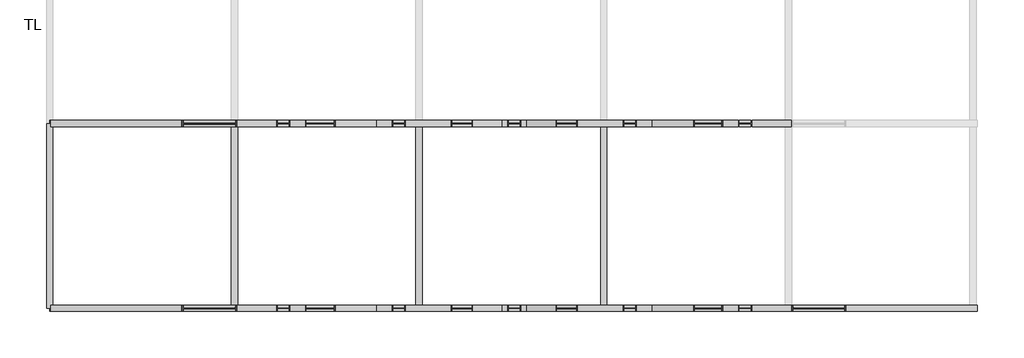
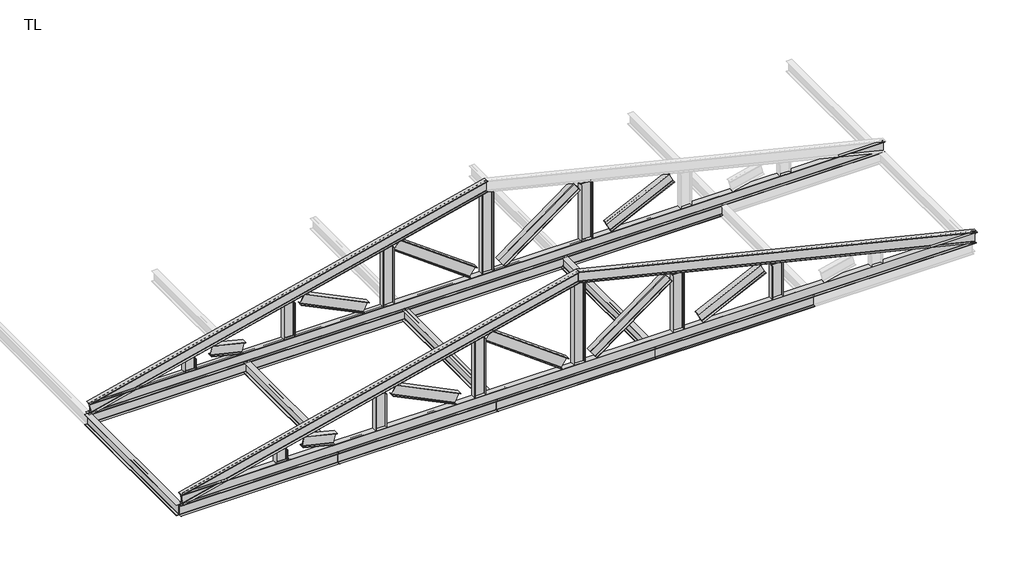
# One storey, part 1 of 4: 38 beams.
"""IFC4 building model written with IfcOpenShell, lengths in millimetres."""

from ifc_helpers import new_model, si_unit, frame, origin, place, context, project, spatial, polyline, circle_curve, ellipse_curve, transform, mapped, element, save
from ifc_brep_helpers import plane_surface, revolved_surface, advanced_brep
from components import w_shapes_w14x30_920474df, w_shapes_w14x30_f0ef5163, w_shapes_w14x30_e8a2e8cf, w_shapes_w14x30_72b19b1b, w_shapes_w14x30_b44ec7f2, w_shapes_w14x30_809da129, w_shapes_w14x30_b6c746c8, w_shapes_w14x30_333ad3b1, w_shapes_w14x30_a113fbeb, w_shapes_w14x30_23e28ad8, w_shapes_w14x30_8f152a7c

model = new_model("IFC4")

# Units and contexts
model_context = context("Model", 3, world=origin())
ifc_project = project(units=[si_unit("LENGTHUNIT", "METRE", prefix="MILLI")], contexts=[model_context])

# Site, building, storey
site = spatial("IfcSite", under=ifc_project)
building = spatial("IfcBuilding", under=site)
storey = spatial("IfcBuildingStorey", under=building, Name="TL", Elevation=8534.4)

# Beams
placement = place(None, origin())
element("IfcBeam", 1, ObjectType="W Shapes : W14X30", at=placement, inside=storey, context=model_context, shape_type="AdvancedBrep", body=[
    advanced_brep(
    [(-18310.2356148, -875.6664521, 8538.7295322), (-18307.9189802, -875.6664521, 8529.2288983), (-18307.9189802, -1046.6084521, 8529.2288983), (-18310.2356148, -1046.6084521, 8538.7295322), (-18310.2356148, -974.7264521, 8538.7295322), (-18312.6425079, -964.5664521, 8548.6003207), (-18386.2332635, -964.5664521, 8850.3996793), (-18388.6401565, -974.7264521, 8860.2704678), (-18388.6401565, -1046.6084521, 8860.2704678), (-18390.9567911, -1046.6084521, 8869.7711017), (-18390.9567911, -875.6664521, 8869.7711017), (-18388.6401565, -875.6664521, 8860.2704678), (-18388.6401565, -947.5484521, 8860.2704678), (-18386.2332635, -957.7084521, 8850.3996793), (-18312.6425079, -957.7084521, 8548.6003207), (-18310.2356148, -947.5484521, 8538.7295322), (-5849.4378857, -947.5484521, 11577.1704505), (-5849.4378857, -875.6664521, 11577.1704505), (-5849.4378857, -957.7084521, 11587.6281358), (-5849.4378857, -957.7084521, 11907.3718642), (-5849.4378857, -947.5484521, 11917.8295495), (-5849.4378857, -875.6664521, 11917.8295495), (-5849.4378857, -875.6664521, 11927.8950717), (-5849.4378857, -1046.6084521, 11927.8950717), (-5849.4378857, -1046.6084521, 11917.8295495), (-5849.4378857, -974.7264521, 11917.8295495), (-5849.4378857, -964.5664521, 11907.3718642), (-5849.4378857, -964.5664521, 11587.6281358), (-5849.4378857, -974.7264521, 11577.1704505), (-5849.4378857, -1046.6084521, 11577.1704505), (-5849.4378857, -1046.6084521, 11567.1049283), (-5849.4378857, -875.6664521, 11567.1049283)],
    [
        (0, 1),
        (1, 2),
        (2, 3),
        (3, 4),
        (4, 5, circle_curve(frame((-18312.6425079, -974.7264521, 8548.6003207), z_axis=(0.971534301878756, 0.0, 0.23689892417011604), x_axis=(0.23689892417011604, 0.0, -0.971534301878756)), 10.16)),
        (5, 6),
        (6, 7, circle_curve(frame((-18386.2332635, -974.7264521, 8850.3996793), z_axis=(0.971534301878756, 0.0, 0.23689892417011604), x_axis=(0.0, 1.0000000000000002, 0.0)), 10.16)),
        (7, 8),
        (8, 9),
        (9, 10),
        (10, 11),
        (11, 12),
        (12, 13, circle_curve(frame((-18386.2332635, -947.5484521, 8850.3996793), z_axis=(0.971534301878756, 0.0, 0.23689892417011604), x_axis=(-0.23689892417011604, 0.0, 0.971534301878756)), 10.16)),
        (13, 14),
        (14, 15, circle_curve(frame((-18312.6425079, -947.5484521, 8548.6003207), z_axis=(0.971534301878756, 0.0, 0.23689892417011604), x_axis=(0.0, -1.0000000000000002, 0.0)), 10.16)),
        (15, 0),
        (16, 17),
        (17, 0),
        (15, 16),
        (18, 16, ellipse_curve(frame((-5849.4378857, -947.5484521, 11587.6281358), z_axis=(1.0, 0.0, 0.0), x_axis=(0.0, 0.0, -1.0)), 10.4576853, 10.16)),
        (14, 18),
        (19, 18),
        (13, 19),
        (20, 19, ellipse_curve(frame((-5849.4378857, -947.5484521, 11907.3718642), z_axis=(1.0, 0.0, 0.0), x_axis=(0.0, 0.0, -1.0)), 10.4576853, 10.16)),
        (12, 20),
        (21, 20),
        (11, 21),
        (22, 21),
        (10, 22),
        (23, 22),
        (9, 23),
        (24, 23),
        (8, 24),
        (25, 24),
        (7, 25),
        (26, 25, ellipse_curve(frame((-5849.4378857, -974.7264521, 11907.3718642), z_axis=(1.0, 0.0, 0.0), x_axis=(0.0, 0.0, -1.0)), 10.4576853, 10.16)),
        (6, 26),
        (27, 26),
        (5, 27),
        (28, 27, ellipse_curve(frame((-5849.4378857, -974.7264521, 11587.6281358), z_axis=(1.0, 0.0, 0.0), x_axis=(0.0, 0.0, -1.0)), 10.4576853, 10.16)),
        (4, 28),
        (29, 28),
        (3, 29),
        (30, 29),
        (2, 30),
        (31, 30),
        (1, 31),
        (17, 31),
    ],
    [
        plane_surface(frame((-18349.4378857, -961.1374521, 8699.5), z_axis=(-0.971534301878756, 0.0, -0.23689892417011604), x_axis=(-0.23689892417011604, 0.0, 0.971534301878756))),
        plane_surface(frame((-5810.2356148, -911.6074521, 11586.7295322), z_axis=(-0.23689892417011604, 0.0, 0.971534301878756), x_axis=(0.0, -1.0, 0.0))),
        revolved_surface(polyline([(-18312.6425079, -957.7084520999999, 8548.600320699998), (-5847.030992628227, -957.7084520999999, 11588.215032583868)]), (-5812.6425079, -947.5484521, 11596.6003207), (-0.971534301878756, 0.0, -0.23689892417011604)),
        plane_surface(frame((-5849.4378857, -957.7084521, 11747.5), z_axis=(0.0, 1.0000000000000002, 0.0), x_axis=(-0.23689892417011604, 0.0, 0.971534301878756))),
        revolved_surface(polyline([(-18388.640156569567, -947.5484521, 8860.270467807088), (-5849.437885708268, -947.5484521, 11917.82954953391)]), (-5886.2332635, -947.5484521, 11898.3996793), (-0.971534301878756, 0.0, -0.23689892417011604)),
        plane_surface(frame((-5888.6401565, -911.6074521, 11908.2704678), z_axis=(0.23689892417011604, 0.0, -0.971534301878756), x_axis=(0.0, 1.0, 0.0))),
        plane_surface(frame((-5889.7984738, -875.6664521, 11913.0207848), z_axis=(0.0, 1.0000000000000002, 0.0), x_axis=(-0.23689892417011604, 0.0, 0.971534301878756))),
        plane_surface(frame((-5890.9567911, -961.1374521, 11917.7711017), z_axis=(-0.23689892417011604, 0.0, 0.971534301878756), x_axis=(0.0, -1.0, 0.0))),
        plane_surface(frame((-5889.7984738, -1046.6084521, 11913.0207848), z_axis=(0.0, -1.0000000000000002, 0.0), x_axis=(0.23689892417011604, 0.0, -0.971534301878756))),
        plane_surface(frame((-5888.6401565, -1010.6674521, 11908.2704678), z_axis=(0.23689892417011604, 0.0, -0.971534301878756), x_axis=(0.0, 1.0, 0.0))),
        revolved_surface(polyline([(-18386.2332635, -964.5664521, 8850.399679299999), (-5847.0309926387, -964.5664521, 11907.95876102682)]), (-5886.2332635, -974.7264521, 11898.3996793), (-0.971534301878756, 0.0, -0.23689892417011604)),
        plane_surface(frame((-5849.4378857, -964.5664521, 11747.5), z_axis=(0.0, -1.0000000000000002, 0.0), x_axis=(0.23689892417011604, 0.0, -0.971534301878756))),
        revolved_surface(polyline([(-18310.23561483043, -974.7264521, 8538.729532192909), (-5844.624099558659, -974.7264521, 11578.34424407678)]), (-5812.6425079, -974.7264521, 11596.6003207), (-0.971534301878756, 0.0, -0.23689892417011604)),
        plane_surface(frame((-5810.2356148, -1010.6674521, 11586.7295322), z_axis=(-0.23689892417011604, 0.0, 0.971534301878756), x_axis=(0.0, -1.0, 0.0))),
        plane_surface(frame((-5809.0772975, -1046.6084521, 11581.9792152), z_axis=(0.0, -1.0000000000000002, 0.0), x_axis=(0.23689892417011604, 0.0, -0.971534301878756))),
        plane_surface(frame((-5807.9189802, -961.1374521, 11577.2288983), z_axis=(0.23689892417011604, 0.0, -0.971534301878756), x_axis=(0.0, 1.0, 0.0))),
        plane_surface(frame((-5809.0772975, -875.6664521, 11581.9792152), z_axis=(0.0, 1.0000000000000002, 0.0), x_axis=(-0.23689892417011604, 0.0, 0.971534301878756))),
        plane_surface(frame((-5849.4378857, -961.1374521, 11927.8950717), z_axis=(1.0, 0.0, 0.0), x_axis=(0.0, -1.0, 0.0))),
    ],
    [
        (0, [[1, 2, 3, 4, 5, 6, 7, 8, 9, 10, 11, 12, 13, 14, 15, 16]]),
        (1, [[17, 18, -16, 19]]),
        (2, [[20, -19, -15, 21]]),
        (3, [[22, -21, -14, 23]]),
        (4, [[24, -23, -13, 25]]),
        (5, [[26, -25, -12, 27]]),
        (6, [[28, -27, -11, 29]]),
        (7, [[30, -29, -10, 31]]),
        (8, [[32, -31, -9, 33]]),
        (9, [[34, -33, -8, 35]]),
        (10, [[36, -35, -7, 37]]),
        (11, [[38, -37, -6, 39]]),
        (12, [[40, -39, -5, 41]]),
        (13, [[42, -41, -4, 43]]),
        (14, [[44, -43, -3, 45]]),
        (15, [[46, -45, -2, 47]]),
        (16, [[48, -47, -1, -18]]),
        (17, [[-17, -20, -22, -24, -26, -28, -30, -32, -34, -36, -38, -40, -42, -44, -46, -48]]),
    ],
),
])
element("IfcBeam", 2, ObjectType="W Shapes : W14X30", at=placement, inside=storey, context=model_context, shape_type="AdvancedBrep", body=[
    advanced_brep(
    [(-18310.2356148, -5875.6664521, 8538.7295322), (-18307.9189802, -5875.6664521, 8529.2288983), (-18307.9189802, -6046.6084521, 8529.2288983), (-18310.2356148, -6046.6084521, 8538.7295322), (-18310.2356148, -5974.7264521, 8538.7295322), (-18312.6425079, -5964.5664521, 8548.6003207), (-18386.2332635, -5964.5664521, 8850.3996793), (-18388.6401565, -5974.7264521, 8860.2704678), (-18388.6401565, -6046.6084521, 8860.2704678), (-18390.9567911, -6046.6084521, 8869.7711017), (-18390.9567911, -5875.6664521, 8869.7711017), (-18388.6401565, -5875.6664521, 8860.2704678), (-18388.6401565, -5947.5484521, 8860.2704678), (-18386.2332635, -5957.7084521, 8850.3996793), (-18312.6425079, -5957.7084521, 8548.6003207), (-18310.2356148, -5947.5484521, 8538.7295322), (-5849.4378857, -5947.5484521, 11577.1704505), (-5849.4378857, -5875.6664521, 11577.1704505), (-5849.4378857, -5957.7084521, 11587.6281358), (-5849.4378857, -5957.7084521, 11907.3718642), (-5849.4378857, -5947.5484521, 11917.8295495), (-5849.4378857, -5875.6664521, 11917.8295495), (-5849.4378857, -5875.6664521, 11927.8950717), (-5849.4378857, -6046.6084521, 11927.8950717), (-5849.4378857, -6046.6084521, 11917.8295495), (-5849.4378857, -5974.7264521, 11917.8295495), (-5849.4378857, -5964.5664521, 11907.3718642), (-5849.4378857, -5964.5664521, 11587.6281358), (-5849.4378857, -5974.7264521, 11577.1704505), (-5849.4378857, -6046.6084521, 11577.1704505), (-5849.4378857, -6046.6084521, 11567.1049283), (-5849.4378857, -5875.6664521, 11567.1049283)],
    [
        (0, 1),
        (1, 2),
        (2, 3),
        (3, 4),
        (4, 5, circle_curve(frame((-18312.6425079, -5974.7264521, 8548.6003207), z_axis=(0.971534301878756, 0.0, 0.23689892417011604), x_axis=(0.23689892417011604, 0.0, -0.971534301878756)), 10.16)),
        (5, 6),
        (6, 7, circle_curve(frame((-18386.2332635, -5974.7264521, 8850.3996793), z_axis=(0.971534301878756, 0.0, 0.23689892417011604), x_axis=(0.0, 1.0000000000000002, 0.0)), 10.16)),
        (7, 8),
        (8, 9),
        (9, 10),
        (10, 11),
        (11, 12),
        (12, 13, circle_curve(frame((-18386.2332635, -5947.5484521, 8850.3996793), z_axis=(0.971534301878756, 0.0, 0.23689892417011604), x_axis=(-0.23689892417011604, 0.0, 0.971534301878756)), 10.16)),
        (13, 14),
        (14, 15, circle_curve(frame((-18312.6425079, -5947.5484521, 8548.6003207), z_axis=(0.971534301878756, 0.0, 0.23689892417011604), x_axis=(0.0, -1.0000000000000002, 0.0)), 10.16)),
        (15, 0),
        (16, 17),
        (17, 0),
        (15, 16),
        (18, 16, ellipse_curve(frame((-5849.4378857, -5947.5484521, 11587.6281358), z_axis=(1.0, 0.0, 0.0), x_axis=(0.0, 0.0, -1.0)), 10.4576853, 10.16)),
        (14, 18),
        (19, 18),
        (13, 19),
        (20, 19, ellipse_curve(frame((-5849.4378857, -5947.5484521, 11907.3718642), z_axis=(1.0, 0.0, 0.0), x_axis=(0.0, 0.0, -1.0)), 10.4576853, 10.16)),
        (12, 20),
        (21, 20),
        (11, 21),
        (22, 21),
        (10, 22),
        (23, 22),
        (9, 23),
        (24, 23),
        (8, 24),
        (25, 24),
        (7, 25),
        (26, 25, ellipse_curve(frame((-5849.4378857, -5974.7264521, 11907.3718642), z_axis=(1.0, 0.0, 0.0), x_axis=(0.0, 0.0, -1.0)), 10.4576853, 10.16)),
        (6, 26),
        (27, 26),
        (5, 27),
        (28, 27, ellipse_curve(frame((-5849.4378857, -5974.7264521, 11587.6281358), z_axis=(1.0, 0.0, 0.0), x_axis=(0.0, 0.0, -1.0)), 10.4576853, 10.16)),
        (4, 28),
        (29, 28),
        (3, 29),
        (30, 29),
        (2, 30),
        (31, 30),
        (1, 31),
        (17, 31),
    ],
    [
        plane_surface(frame((-18349.4378857, -5961.1374521, 8699.5), z_axis=(-0.971534301878756, 0.0, -0.23689892417011604), x_axis=(-0.23689892417011604, 0.0, 0.971534301878756))),
        plane_surface(frame((-5810.2356148, -5911.6074521, 11586.7295322), z_axis=(-0.23689892417011604, 0.0, 0.971534301878756), x_axis=(0.0, -1.0, 0.0))),
        revolved_surface(polyline([(-18312.6425079, -5957.7084521, 8548.600320699998), (-5847.030992628227, -5957.7084521, 11588.215032583868)]), (-5812.6425079, -5947.5484521, 11596.6003207), (-0.971534301878756, 0.0, -0.23689892417011604)),
        plane_surface(frame((-5849.4378857, -5957.7084521, 11747.5), z_axis=(0.0, 1.0000000000000002, 0.0), x_axis=(-0.23689892417011604, 0.0, 0.971534301878756))),
        revolved_surface(polyline([(-18388.640156569567, -5947.5484521, 8860.270467807088), (-5849.437885708268, -5947.5484521, 11917.82954953391)]), (-5886.2332635, -5947.5484521, 11898.3996793), (-0.971534301878756, 0.0, -0.23689892417011604)),
        plane_surface(frame((-5888.6401565, -5911.6074521, 11908.2704678), z_axis=(0.23689892417011604, 0.0, -0.971534301878756), x_axis=(0.0, 1.0, 0.0))),
        plane_surface(frame((-5889.7984738, -5875.6664521, 11913.0207848), z_axis=(0.0, 1.0000000000000002, 0.0), x_axis=(-0.23689892417011604, 0.0, 0.971534301878756))),
        plane_surface(frame((-5890.9567911, -5961.1374521, 11917.7711017), z_axis=(-0.23689892417011604, 0.0, 0.971534301878756), x_axis=(0.0, -1.0, 0.0))),
        plane_surface(frame((-5889.7984738, -6046.6084521, 11913.0207848), z_axis=(0.0, -1.0000000000000002, 0.0), x_axis=(0.23689892417011604, 0.0, -0.971534301878756))),
        plane_surface(frame((-5888.6401565, -6010.6674521, 11908.2704678), z_axis=(0.23689892417011604, 0.0, -0.971534301878756), x_axis=(0.0, 1.0, 0.0))),
        revolved_surface(polyline([(-18386.2332635, -5964.5664521, 8850.399679299999), (-5847.0309926387, -5964.5664521, 11907.95876102682)]), (-5886.2332635, -5974.7264521, 11898.3996793), (-0.971534301878756, 0.0, -0.23689892417011604)),
        plane_surface(frame((-5849.4378857, -5964.5664521, 11747.5), z_axis=(0.0, -1.0000000000000002, 0.0), x_axis=(0.23689892417011604, 0.0, -0.971534301878756))),
        revolved_surface(polyline([(-18310.23561483043, -5974.7264521, 8538.729532192909), (-5844.624099558659, -5974.7264521, 11578.34424407678)]), (-5812.6425079, -5974.7264521, 11596.6003207), (-0.971534301878756, 0.0, -0.23689892417011604)),
        plane_surface(frame((-5810.2356148, -6010.6674521, 11586.7295322), z_axis=(-0.23689892417011604, 0.0, 0.971534301878756), x_axis=(0.0, -1.0, 0.0))),
        plane_surface(frame((-5809.0772975, -6046.6084521, 11581.9792152), z_axis=(0.0, -1.0000000000000002, 0.0), x_axis=(0.23689892417011604, 0.0, -0.971534301878756))),
        plane_surface(frame((-5807.9189802, -5961.1374521, 11577.2288983), z_axis=(0.23689892417011604, 0.0, -0.971534301878756), x_axis=(0.0, 1.0, 0.0))),
        plane_surface(frame((-5809.0772975, -5875.6664521, 11581.9792152), z_axis=(0.0, 1.0000000000000002, 0.0), x_axis=(-0.23689892417011604, 0.0, 0.971534301878756))),
        plane_surface(frame((-5849.4378857, -5961.1374521, 11927.8950717), z_axis=(1.0, 0.0, 0.0), x_axis=(0.0, -1.0, 0.0))),
    ],
    [
        (0, [[1, 2, 3, 4, 5, 6, 7, 8, 9, 10, 11, 12, 13, 14, 15, 16]]),
        (1, [[17, 18, -16, 19]]),
        (2, [[20, -19, -15, 21]]),
        (3, [[22, -21, -14, 23]]),
        (4, [[24, -23, -13, 25]]),
        (5, [[26, -25, -12, 27]]),
        (6, [[28, -27, -11, 29]]),
        (7, [[30, -29, -10, 31]]),
        (8, [[32, -31, -9, 33]]),
        (9, [[34, -33, -8, 35]]),
        (10, [[36, -35, -7, 37]]),
        (11, [[38, -37, -6, 39]]),
        (12, [[40, -39, -5, 41]]),
        (13, [[42, -41, -4, 43]]),
        (14, [[44, -43, -3, 45]]),
        (15, [[46, -45, -2, 47]]),
        (16, [[48, -47, -1, -18]]),
        (17, [[-17, -20, -22, -24, -26, -28, -30, -32, -34, -36, -38, -40, -42, -44, -46, -48]]),
    ],
),
])
element("IfcBeam", 3, ObjectType="W Shapes : W14X30", at=placement, inside=storey, context=model_context, shape_type="AdvancedBrep", body=[
    advanced_brep(
    [(6611.3598435, -5875.6664521, 8538.7295322), (6611.3598435, -5947.5484521, 8538.7295322), (6613.7667365, -5957.7084521, 8548.6003207), (6687.3574921, -5957.7084521, 8850.3996793), (6689.7643852, -5947.5484521, 8860.2704678), (6689.7643852, -5875.6664521, 8860.2704678), (6692.0810198, -5875.6664521, 8869.7711017), (6692.0810198, -6046.6084521, 8869.7711017), (6689.7643852, -6046.6084521, 8860.2704678), (6689.7643852, -5974.7264521, 8860.2704678), (6687.3574921, -5964.5664521, 8850.3996793), (6613.7667365, -5964.5664521, 8548.6003207), (6611.3598435, -5974.7264521, 8538.7295322), (6611.3598435, -6046.6084521, 8538.7295322), (6609.0432089, -6046.6084521, 8529.2288983), (6609.0432089, -5875.6664521, 8529.2288983), (-5849.4378857, -5875.6664521, 11577.1704505), (-5849.4378857, -5947.5484521, 11577.1704505), (-5849.4378857, -5957.7084521, 11587.6281358), (-5849.4378857, -5957.7084521, 11907.3718642), (-5849.4378857, -5947.5484521, 11917.8295495), (-5849.4378857, -5875.6664521, 11917.8295495), (-5849.4378857, -5875.6664521, 11927.8950717), (-5849.4378857, -6046.6084521, 11927.8950717), (-5849.4378857, -6046.6084521, 11917.8295495), (-5849.4378857, -5974.7264521, 11917.8295495), (-5849.4378857, -5964.5664521, 11907.3718642), (-5849.4378857, -5964.5664521, 11587.6281358), (-5849.4378857, -5974.7264521, 11577.1704505), (-5849.4378857, -6046.6084521, 11577.1704505), (-5849.4378857, -6046.6084521, 11567.1049283), (-5849.4378857, -5875.6664521, 11567.1049283)],
    [
        (0, 1),
        (1, 2, circle_curve(frame((6613.7667365, -5947.5484521, 8548.6003207), z_axis=(-0.971534301878756, 0.0, 0.23689892417011588), x_axis=(0.0, -1.0, 0.0)), 10.16)),
        (2, 3),
        (3, 4, circle_curve(frame((6687.3574921, -5947.5484521, 8850.3996793), z_axis=(-0.971534301878756, 0.0, 0.23689892417011588), x_axis=(0.23689892417011588, 0.0, 0.971534301878756)), 10.16)),
        (4, 5),
        (5, 6),
        (6, 7),
        (7, 8),
        (8, 9),
        (9, 10, circle_curve(frame((6687.3574921, -5974.7264521, 8850.3996793), z_axis=(-0.971534301878756, 0.0, 0.23689892417011588), x_axis=(0.0, 1.0, 0.0)), 10.16)),
        (10, 11),
        (11, 12, circle_curve(frame((6613.7667365, -5974.7264521, 8548.6003207), z_axis=(-0.971534301878756, 0.0, 0.23689892417011588), x_axis=(-0.23689892417011588, 0.0, -0.971534301878756)), 10.16)),
        (12, 13),
        (13, 14),
        (14, 15),
        (15, 0),
        (0, 16),
        (16, 17),
        (17, 1),
        (17, 18, ellipse_curve(frame((-5849.4378857, -5947.5484521, 11587.6281358), z_axis=(-1.0, 0.0, 0.0), x_axis=(0.0, 0.0, 1.0)), 10.4576853, 10.16)),
        (18, 2),
        (18, 19),
        (19, 3),
        (19, 20, ellipse_curve(frame((-5849.4378857, -5947.5484521, 11907.3718642), z_axis=(-1.0, 0.0, 0.0), x_axis=(0.0, 0.0, 1.0)), 10.4576853, 10.16)),
        (20, 4),
        (20, 21),
        (21, 5),
        (21, 22),
        (22, 6),
        (22, 23),
        (23, 7),
        (23, 24),
        (24, 8),
        (24, 25),
        (25, 9),
        (25, 26, ellipse_curve(frame((-5849.4378857, -5974.7264521, 11907.3718642), z_axis=(-1.0, 0.0, 0.0), x_axis=(0.0, 0.0, 1.0)), 10.4576853, 10.16)),
        (26, 10),
        (26, 27),
        (27, 11),
        (27, 28, ellipse_curve(frame((-5849.4378857, -5974.7264521, 11587.6281358), z_axis=(-1.0, 0.0, 0.0), x_axis=(0.0, 0.0, 1.0)), 10.4576853, 10.16)),
        (28, 12),
        (28, 29),
        (29, 13),
        (29, 30),
        (30, 14),
        (30, 31),
        (31, 15),
        (31, 16),
    ],
    [
        plane_surface(frame((6650.5621143, -5961.1374521, 8699.5), z_axis=(0.971534301878756, 0.0, -0.23689892417011588), x_axis=(0.23689892417011588, 0.0, 0.971534301878756))),
        plane_surface(frame((6611.3598435, -5911.6074521, 8538.7295322), z_axis=(0.23689892417011588, 0.0, 0.971534301878756), x_axis=(0.0, -1.0, 0.0))),
        revolved_surface(polyline([(-5851.844778771774, -5957.7084521, 11588.215032583868), (6613.766736564033, -5957.7084521, 8548.600320684385)]), (6613.7667365, -5947.5484521, 8548.6003207), (-0.971534301878756, 0.0, 0.23689892417011588)),
        plane_surface(frame((6650.5621143, -5957.7084521, 8699.5), z_axis=(0.0, 1.0, 0.0), x_axis=(0.23689892417011588, 0.0, 0.971534301878756))),
        revolved_surface(polyline([(-5849.437885691734, -5947.5484521, 11917.82954953391), (6689.764385199924, -5947.5484521, 8860.270467799688)]), (6687.3574921, -5947.5484521, 8850.3996793), (-0.971534301878756, 0.0, 0.23689892417011588)),
        plane_surface(frame((6689.7643852, -5911.6074521, 8860.2704678), z_axis=(-0.23689892417011588, 0.0, -0.971534301878756), x_axis=(0.0, 1.0, 0.0))),
        plane_surface(frame((6690.9227025, -5875.6664521, 8865.0207848), z_axis=(0.0, 1.0, 0.0), x_axis=(0.23689892417011588, 0.0, 0.971534301878756))),
        plane_surface(frame((6692.0810198, -5961.1374521, 8869.7711017), z_axis=(0.23689892417011588, 0.0, 0.971534301878756), x_axis=(0.0, -1.0, 0.0))),
        plane_surface(frame((6690.9227025, -6046.6084521, 8865.0207848), z_axis=(0.0, -1.0, 0.0), x_axis=(-0.23689892417011588, 0.0, -0.971534301878756))),
        plane_surface(frame((6689.7643852, -6010.6674521, 8860.2704678), z_axis=(-0.23689892417011588, 0.0, -0.971534301878756), x_axis=(0.0, 1.0, 0.0))),
        revolved_surface(polyline([(-5851.844778761302, -5964.5664521, 11907.95876102682), (6687.357492130355, -5964.5664521, 8850.3996792926)]), (6687.3574921, -5974.7264521, 8850.3996793), (-0.971534301878756, 0.0, 0.23689892417011588)),
        plane_surface(frame((6650.5621143, -5964.5664521, 8699.5), z_axis=(0.0, -1.0, 0.0), x_axis=(-0.23689892417011588, 0.0, -0.971534301878756))),
        revolved_surface(polyline([(-5854.251671841343, -5974.7264521, 11578.34424407678), (6611.359843494464, -5974.7264521, 8538.729532177296)]), (6613.7667365, -5974.7264521, 8548.6003207), (-0.971534301878756, 0.0, 0.23689892417011588)),
        plane_surface(frame((6611.3598435, -6010.6674521, 8538.7295322), z_axis=(0.23689892417011588, 0.0, 0.971534301878756), x_axis=(0.0, -1.0, 0.0))),
        plane_surface(frame((6610.2015262, -6046.6084521, 8533.9792152), z_axis=(0.0, -1.0, 0.0), x_axis=(-0.23689892417011588, 0.0, -0.971534301878756))),
        plane_surface(frame((6609.0432089, -5961.1374521, 8529.2288983), z_axis=(-0.23689892417011588, 0.0, -0.971534301878756), x_axis=(0.0, 1.0, 0.0))),
        plane_surface(frame((6610.2015262, -5875.6664521, 8533.9792152), z_axis=(0.0, 1.0, 0.0), x_axis=(0.23689892417011588, 0.0, 0.971534301878756))),
        plane_surface(frame((-5849.4378857, -5961.1374521, 11927.8950717), z_axis=(-1.0, 0.0, 0.0), x_axis=(0.0, 1.0, 0.0))),
    ],
    [
        (0, [[1, 2, 3, 4, 5, 6, 7, 8, 9, 10, 11, 12, 13, 14, 15, 16]]),
        (1, [[-1, 17, 18, 19]]),
        (2, [[-2, -19, 20, 21]]),
        (3, [[-3, -21, 22, 23]]),
        (4, [[-4, -23, 24, 25]]),
        (5, [[-5, -25, 26, 27]]),
        (6, [[-6, -27, 28, 29]]),
        (7, [[-7, -29, 30, 31]]),
        (8, [[-8, -31, 32, 33]]),
        (9, [[-9, -33, 34, 35]]),
        (10, [[-10, -35, 36, 37]]),
        (11, [[-11, -37, 38, 39]]),
        (12, [[-12, -39, 40, 41]]),
        (13, [[-13, -41, 42, 43]]),
        (14, [[-14, -43, 44, 45]]),
        (15, [[-15, -45, 46, 47]]),
        (16, [[-16, -47, 48, -17]]),
        (17, [[-48, -46, -44, -42, -40, -38, -36, -34, -32, -30, -28, -26, -24, -22, -20, -18]]),
    ],
),
])
w_shapes_w14x30_shape = w_shapes_w14x30_920474df(model_context)
element("IfcBeam", 4, ObjectType="W Shapes : W14X30", at=placement, inside=storey, context=model_context, shape_type="MappedRepresentation", body=[
    mapped(w_shapes_w14x30_shape, transform((-15925.6378857, -5961.1374521, 8359.14), x_axis=(1.0, 0.0, 0.0), y_axis=(0.0, 1.0, 0.0), z_axis=(0.0, 0.0, 1.0))),
])
element("IfcBeam", 5, ObjectType="W Shapes : W14X30", at=placement, inside=storey, context=model_context, shape_type="MappedRepresentation", body=[
    mapped(w_shapes_w14x30_shape, transform((-10925.6378857, -5961.1374521, 8359.14), x_axis=(1.0, 0.0, 0.0), y_axis=(0.0, 1.0, 0.0), z_axis=(0.0, 0.0, 1.0))),
])
element("IfcBeam", 6, ObjectType="W Shapes : W14X30", at=placement, inside=storey, context=model_context, shape_type="MappedRepresentation", body=[
    mapped(w_shapes_w14x30_shape, transform((-5925.6378857, -5961.1374521, 8359.14), x_axis=(1.0, 0.0, 0.0), y_axis=(0.0, 1.0, 0.0), z_axis=(0.0, 0.0, 1.0))),
])
element("IfcBeam", 7, ObjectType="W Shapes : W14X30", at=placement, inside=storey, context=model_context, shape_type="MappedRepresentation", body=[
    mapped(w_shapes_w14x30_shape, transform((-925.6378857, -5961.1374521, 8359.14), x_axis=(1.0, 0.0, 0.0), y_axis=(0.0, 1.0, 0.0), z_axis=(0.0, 0.0, 1.0))),
])
element("IfcBeam", 8, ObjectType="W Shapes : W14X30", at=placement, inside=storey, context=model_context, shape_type="MappedRepresentation", body=[
    mapped(w_shapes_w14x30_shape, transform((-15925.6378857, -961.1374521, 8359.14), x_axis=(1.0, 0.0, 0.0), y_axis=(0.0, 1.0, 0.0), z_axis=(0.0, 0.0, 1.0))),
])
element("IfcBeam", 9, ObjectType="W Shapes : W14X30", at=placement, inside=storey, context=model_context, shape_type="MappedRepresentation", body=[
    mapped(w_shapes_w14x30_shape, transform((-10925.6378857, -961.1374521, 8359.14), x_axis=(1.0, 0.0, 0.0), y_axis=(0.0, 1.0, 0.0), z_axis=(0.0, 0.0, 1.0))),
])
element("IfcBeam", 10, ObjectType="W Shapes : W14X30", at=placement, inside=storey, context=model_context, shape_type="MappedRepresentation", body=[
    mapped(w_shapes_w14x30_shape, transform((-5925.6378857, -961.1374521, 8359.14), x_axis=(1.0, 0.0, 0.0), y_axis=(0.0, 1.0, 0.0), z_axis=(0.0, 0.0, 1.0))),
])
element("IfcBeam", 11, ObjectType="W Shapes : W14X30", at=placement, inside=storey, context=model_context, shape_type="MappedRepresentation", body=[
    mapped(w_shapes_w14x30_shape, transform((-925.6378857, -961.1374521, 8359.14), x_axis=(1.0, 0.0, 0.0), y_axis=(0.0, 1.0, 0.0), z_axis=(0.0, 0.0, 1.0))),
])
element("IfcBeam", 12, ObjectType="W Shapes : W14X30", at=placement, inside=storey, context=model_context, shape_type="MappedRepresentation", body=[
    mapped(w_shapes_w14x30_shape, transform((-3425.6378857, -3461.1374521, 8359.14), x_axis=(0.0, 1.0, 0.0), y_axis=(-1.0, 0.0, 0.0), z_axis=(0.0, 0.0, 1.0))),
])
element("IfcBeam", 13, ObjectType="W Shapes : W14X30", at=placement, inside=storey, context=model_context, shape_type="MappedRepresentation", body=[
    mapped(w_shapes_w14x30_shape, transform((-8425.6378857, -3461.1374521, 8359.14), x_axis=(0.0, 1.0, 0.0), y_axis=(-1.0, 0.0, 0.0), z_axis=(0.0, 0.0, 1.0))),
])
element("IfcBeam", 14, ObjectType="W Shapes : W14X30", at=placement, inside=storey, context=model_context, shape_type="MappedRepresentation", body=[
    mapped(w_shapes_w14x30_shape, transform((-13425.6378857, -3461.1374521, 8359.14), x_axis=(0.0, 1.0, 0.0), y_axis=(-1.0, 0.0, 0.0), z_axis=(0.0, 0.0, 1.0))),
])
element("IfcBeam", 15, ObjectType="W Shapes : W14X30", at=placement, inside=storey, context=model_context, shape_type="MappedRepresentation", body=[
    mapped(w_shapes_w14x30_shape, transform((-18425.6378857, -3461.1374521, 8359.14), x_axis=(0.0, 1.0, 0.0), y_axis=(-1.0, 0.0, 0.0), z_axis=(0.0, 0.0, 1.0))),
])
w_shapes_w14x30_2_shape = w_shapes_w14x30_f0ef5163(model_context)
element("IfcBeam", 16, ObjectType="W Shapes : W14X30", at=placement, inside=storey, context=model_context, shape_type="MappedRepresentation", body=[
    mapped(w_shapes_w14x30_2_shape, transform((-5849.4378857, -961.1374521, 8699.5), x_axis=(1.0, 0.0, 0.0), y_axis=(0.0, 1.0, 0.0), z_axis=(0.0, 0.0, 1.0))),
])
element("IfcBeam", 17, ObjectType="W Shapes : W14X30", at=placement, inside=storey, context=model_context, shape_type="MappedRepresentation", body=[
    mapped(w_shapes_w14x30_2_shape, transform((-5849.4378857, -5961.1374521, 8699.5), x_axis=(1.0, 0.0, 0.0), y_axis=(0.0, 1.0, 0.0), z_axis=(0.0, 0.0, 1.0))),
])
w_shapes_w14x30_3_shape = w_shapes_w14x30_e8a2e8cf(model_context)
element("IfcBeam", 18, ObjectType="W Shapes : W14X30", at=placement, inside=storey, context=model_context, shape_type="MappedRepresentation", body=[
    mapped(w_shapes_w14x30_3_shape, transform((-5849.4378857, -961.1374521, 10223.5), x_axis=(0.0, 0.0, 1.0), y_axis=(0.0, -1.0, 0.0), z_axis=(1.0, 0.0, 0.0))),
])
element("IfcBeam", 19, ObjectType="W Shapes : W14X30", at=placement, inside=storey, context=model_context, shape_type="MappedRepresentation", body=[
    mapped(w_shapes_w14x30_3_shape, transform((-5849.4378857, -5961.1374521, 10223.5), x_axis=(0.0, 0.0, 1.0), y_axis=(0.0, -1.0, 0.0), z_axis=(1.0, 0.0, 0.0))),
])
w_shapes_w14x30_4_shape = w_shapes_w14x30_72b19b1b(model_context)
element("IfcBeam", 20, ObjectType="W Shapes : W14X30", at=placement, inside=storey, context=model_context, shape_type="MappedRepresentation", body=[
    mapped(w_shapes_w14x30_4_shape, transform((-8974.4378857, -961.1374521, 9842.5), x_axis=(0.0, 0.0, 1.0), y_axis=(0.0, -1.0, 0.0), z_axis=(1.0, 0.0, 0.0))),
])
element("IfcBeam", 21, ObjectType="W Shapes : W14X30", at=placement, inside=storey, context=model_context, shape_type="MappedRepresentation", body=[
    mapped(w_shapes_w14x30_4_shape, transform((-2724.4378857, -961.1374521, 9842.5), x_axis=(0.0, 0.0, 1.0), y_axis=(0.0, -1.0, 0.0), z_axis=(1.0, 0.0, 0.0))),
])
element("IfcBeam", 22, ObjectType="W Shapes : W14X30", at=placement, inside=storey, context=model_context, shape_type="MappedRepresentation", body=[
    mapped(w_shapes_w14x30_4_shape, transform((-8974.4378857, -5961.1374521, 9842.5), x_axis=(0.0, 0.0, 1.0), y_axis=(0.0, -1.0, 0.0), z_axis=(1.0, 0.0, 0.0))),
])
element("IfcBeam", 23, ObjectType="W Shapes : W14X30", at=placement, inside=storey, context=model_context, shape_type="MappedRepresentation", body=[
    mapped(w_shapes_w14x30_4_shape, transform((-2724.4378857, -5961.1374521, 9842.5), x_axis=(0.0, 0.0, 1.0), y_axis=(0.0, -1.0, 0.0), z_axis=(1.0, 0.0, 0.0))),
])
w_shapes_w14x30_5_shape = w_shapes_w14x30_b44ec7f2(model_context)
element("IfcBeam", 24, ObjectType="W Shapes : W14X30", at=placement, inside=storey, context=model_context, shape_type="MappedRepresentation", body=[
    mapped(w_shapes_w14x30_5_shape, transform((-12099.4378857, -961.1374521, 9461.5), x_axis=(0.0, 0.0, 1.0), y_axis=(0.0, -1.0, 0.0), z_axis=(1.0, 0.0, 0.0))),
])
element("IfcBeam", 25, ObjectType="W Shapes : W14X30", at=placement, inside=storey, context=model_context, shape_type="MappedRepresentation", body=[
    mapped(w_shapes_w14x30_5_shape, transform((-12099.4378857, -5961.1374521, 9461.5), x_axis=(0.0, 0.0, 1.0), y_axis=(0.0, -1.0, 0.0), z_axis=(1.0, 0.0, 0.0))),
])
element("IfcBeam", 26, ObjectType="W Shapes : W14X30", at=placement, inside=storey, context=model_context, shape_type="MappedRepresentation", body=[
    mapped(w_shapes_w14x30_5_shape, transform((400.5621143, -5961.1374521, 9461.5), x_axis=(0.0, 0.0, 1.0), y_axis=(0.0, -1.0, 0.0), z_axis=(1.0, 0.0, 0.0))),
])
w_shapes_w14x30_6_shape = w_shapes_w14x30_809da129(model_context)
element("IfcBeam", 27, ObjectType="W Shapes : W14X30", at=placement, inside=storey, context=model_context, shape_type="MappedRepresentation", body=[
    mapped(w_shapes_w14x30_6_shape, transform((-15224.4378857, -961.1374521, 9080.5), x_axis=(0.0, 0.0, 1.0), y_axis=(0.0, -1.0, 0.0), z_axis=(1.0, 0.0, 0.0))),
])
element("IfcBeam", 28, ObjectType="W Shapes : W14X30", at=placement, inside=storey, context=model_context, shape_type="MappedRepresentation", body=[
    mapped(w_shapes_w14x30_6_shape, transform((-15224.4378857, -5961.1374521, 9080.5), x_axis=(0.0, 0.0, 1.0), y_axis=(0.0, -1.0, 0.0), z_axis=(1.0, 0.0, 0.0))),
])
w_shapes_w14x30_7_shape = w_shapes_w14x30_b6c746c8(model_context)
element("IfcBeam", 29, ObjectType="W Shapes : W14X30", at=placement, inside=storey, context=model_context, shape_type="MappedRepresentation", body=[
    mapped(w_shapes_w14x30_7_shape, transform((-7411.9378857, -961.1374521, 9842.5), x_axis=(0.8071023678442881, 0.0, -0.5904115241254555), y_axis=(0.0, -1.0, 0.0), z_axis=(-0.5904115241254555, 0.0, -0.8071023678442881))),
])
element("IfcBeam", 30, ObjectType="W Shapes : W14X30", at=placement, inside=storey, context=model_context, shape_type="MappedRepresentation", body=[
    mapped(w_shapes_w14x30_7_shape, transform((-7411.9378857, -5961.1374521, 9842.5), x_axis=(0.8071023678442881, 0.0, -0.5904115241254555), y_axis=(0.0, -1.0, 0.0), z_axis=(-0.5904115241254555, 0.0, -0.8071023678442881))),
])
w_shapes_w14x30_8_shape = w_shapes_w14x30_333ad3b1(model_context)
element("IfcBeam", 31, ObjectType="W Shapes : W14X30", at=placement, inside=storey, context=model_context, shape_type="MappedRepresentation", body=[
    mapped(w_shapes_w14x30_8_shape, transform((-10536.9378857, -961.1374521, 9461.5), x_axis=(0.8988126690463005, 0.0, -0.4383329624405008), y_axis=(0.0, -1.0, 0.0), z_axis=(-0.4383329624405008, 0.0, -0.8988126690463005))),
])
element("IfcBeam", 32, ObjectType="W Shapes : W14X30", at=placement, inside=storey, context=model_context, shape_type="MappedRepresentation", body=[
    mapped(w_shapes_w14x30_8_shape, transform((-10536.9378857, -5961.1374521, 9461.5), x_axis=(0.8988126690463005, 0.0, -0.4383329624405008), y_axis=(0.0, -1.0, 0.0), z_axis=(-0.4383329624405008, 0.0, -0.8988126690463005))),
])
w_shapes_w14x30_9_shape = w_shapes_w14x30_a113fbeb(model_context)
element("IfcBeam", 33, ObjectType="W Shapes : W14X30", at=placement, inside=storey, context=model_context, shape_type="MappedRepresentation", body=[
    mapped(w_shapes_w14x30_9_shape, transform((-4286.9378857, -961.1374521, 9842.5), x_axis=(0.8071023678442877, 0.0, 0.590411524125456), y_axis=(0.0, -1.0, 0.0), z_axis=(0.590411524125456, 0.0, -0.8071023678442877))),
])
element("IfcBeam", 34, ObjectType="W Shapes : W14X30", at=placement, inside=storey, context=model_context, shape_type="MappedRepresentation", body=[
    mapped(w_shapes_w14x30_9_shape, transform((-4286.9378857, -5961.1374521, 9842.5), x_axis=(0.8071023678442877, 0.0, 0.590411524125456), y_axis=(0.0, -1.0, 0.0), z_axis=(0.590411524125456, 0.0, -0.8071023678442877))),
])
w_shapes_w14x30_10_shape = w_shapes_w14x30_23e28ad8(model_context)
element("IfcBeam", 35, ObjectType="W Shapes : W14X30", at=placement, inside=storey, context=model_context, shape_type="MappedRepresentation", body=[
    mapped(w_shapes_w14x30_10_shape, transform((-1161.9378857, -961.1374521, 9461.5), x_axis=(0.8988126690463014, 0.0, 0.4383329624404991), y_axis=(0.0, -1.0, 0.0), z_axis=(0.4383329624404991, 0.0, -0.8988126690463014))),
])
element("IfcBeam", 36, ObjectType="W Shapes : W14X30", at=placement, inside=storey, context=model_context, shape_type="MappedRepresentation", body=[
    mapped(w_shapes_w14x30_10_shape, transform((-1161.9378857, -5961.1374521, 9461.5), x_axis=(0.8988126690463014, 0.0, 0.4383329624404991), y_axis=(0.0, -1.0, 0.0), z_axis=(0.4383329624404991, 0.0, -0.8988126690463014))),
])
w_shapes_w14x30_11_shape = w_shapes_w14x30_8f152a7c(model_context)
element("IfcBeam", 37, ObjectType="W Shapes : W14X30", at=placement, inside=storey, context=model_context, shape_type="MappedRepresentation", body=[
    mapped(w_shapes_w14x30_11_shape, transform((-13661.9378857, -961.1374521, 9080.5), x_axis=(0.9715343018787559, 0.0, -0.23689892417011585), y_axis=(0.0, -1.0, 0.0), z_axis=(-0.23689892417011585, 0.0, -0.9715343018787559))),
])
element("IfcBeam", 38, ObjectType="W Shapes : W14X30", at=placement, inside=storey, context=model_context, shape_type="MappedRepresentation", body=[
    mapped(w_shapes_w14x30_11_shape, transform((-13661.9378857, -5961.1374521, 9080.5), x_axis=(0.9715343018787559, 0.0, -0.23689892417011585), y_axis=(0.0, -1.0, 0.0), z_axis=(-0.23689892417011585, 0.0, -0.9715343018787559))),
])

save(model, "model.ifc")

# Revit data of these elements
# Type "W Shapes : W14X30"
#   Section Name Key = "W14X30"
#   Width = 6.730"
#   Web Thickness = 0.270"
#   Web Fillet = 0.400"
#   Warping Constant = 887.00 in⁶
#   Torsional Moment of Inertia = 0.38 in⁴
#   Section Area = 8.85 in²
#   Plastic Modulus weak axis = 8.99 in³
#   Plastic Modulus strong axis = 47.30 in³
#   Perimeter = 4.441 ft²/ft
#   Nominal Weight = 30.00 lbf/ft
#   Moment of Inertia weak axis = 19.60 in⁴
#   Moment of Inertia strong axis = 291.00 in⁴
#   Height = 13.800"
#   Flange Thickness = 0.385"
#   Elastic Modulus weak axis = 5.82 in³
#   Elastic Modulus strong axis = 42.00 in³
#   Clear Web Height = 0' - 11 5/8"
#   Centroid Vertical = 6.900"
#   Centroid Horizontal = 3.365"
#   Bolt Spacing = 0' - 3 1/2"
#   Length [instance default] = 1524 mm
#   Structural Material [instance default] = Steel ASTM A992
#   Principal Axes Angle = 0
# Elements 1, 2, 3 (IfcBeam, "W Shapes : W14X30")
#   Length = 12866.247 mm
#   Structural Material = Steel ASTM A992
#   Phase Created = New Construction
#   Materials on its faces: "Steel ASTM A992"
# Elements 4, 5, 6, 7, 8, 9, 10, 11, 12, 13, 14, 15 (IfcBeam, "W Shapes : W14X30")
#   Length = 5000 mm
#   Structural Material = Steel ASTM A992
#   Phase Created = New Construction
#   Materials on its faces: "Steel ASTM A992"
# Elements 16, 17 (IfcBeam, "W Shapes : W14X30")
#   Length = 25000 mm
#   Structural Material = Steel ASTM A992
#   Phase Created = New Construction
#   Materials on its faces: "Steel ASTM A992"
# Elements 18, 19 (IfcBeam, "W Shapes : W14X30")
#   Length = 3048 mm
#   Structural Material = Steel ASTM A992
#   Phase Created = New Construction
#   Materials on its faces: "Steel ASTM A992"
# Elements 20, 21, 22, 23 (IfcBeam, "W Shapes : W14X30")
#   Length = 2286 mm
#   Structural Material = Steel ASTM A992
#   Phase Created = New Construction
#   Materials on its faces: "Steel ASTM A992"
# Elements 24, 25, 26 (IfcBeam, "W Shapes : W14X30")
#   Length = 1524 mm
#   Structural Material = Steel ASTM A992
#   Phase Created = New Construction
#   Materials on its faces: "Steel ASTM A992"
# Elements 27, 28 (IfcBeam, "W Shapes : W14X30")
#   Length = 762 mm
#   Structural Material = Steel ASTM A992
#   Phase Created = New Construction
#   Materials on its faces: "Steel ASTM A992"
# Elements 29, 30, 33, 34 (IfcBeam, "W Shapes : W14X30")
#   Length = 3871.876 mm
#   Structural Material = Steel ASTM A992
#   Phase Created = New Construction
#   Materials on its faces: "Steel ASTM A992"
# Elements 31, 32, 35, 36 (IfcBeam, "W Shapes : W14X30")
#   Length = 3476.809 mm
#   Structural Material = Steel ASTM A992
#   Phase Created = New Construction
#   Materials on its faces: "Steel ASTM A992"
# Elements 37, 38 (IfcBeam, "W Shapes : W14X30")
#   Length = 3216.562 mm
#   Structural Material = Steel ASTM A992
#   Phase Created = New Construction
#   Materials on its faces: "Steel ASTM A992"
# Materials
#   "Steel ASTM A992": class "Metal", colour RGB 199 199 199, transparency 0, Description = "Structural steel 50ksi", Cost = 0
